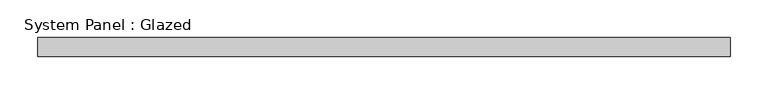
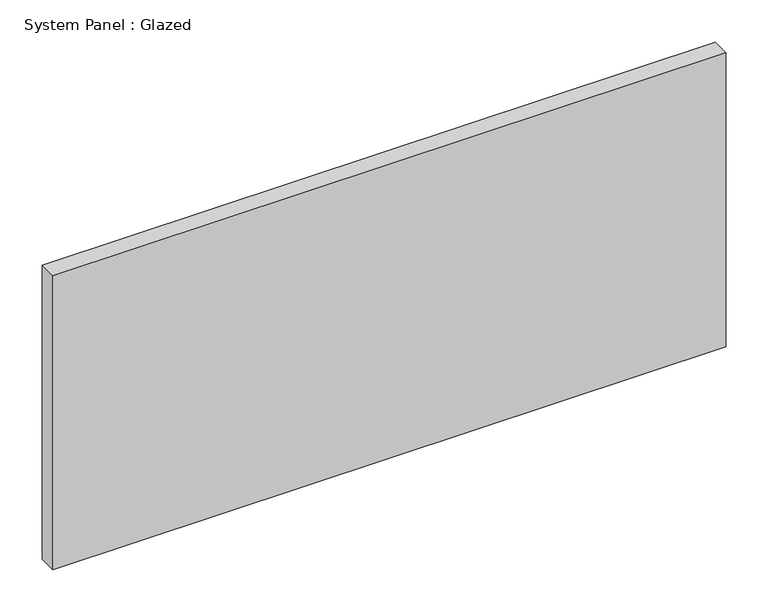
"""IFC4 building model written with IfcOpenShell, lengths in millimetres: plate geometry, System Panel : Glazed."""

from ifc_helpers import new_model, si_unit, origin, origin_with_axes, place, context, project, spatial, polyline, outline, extrude, source, transform, mapped, element, save


def system_panel_glazed_5efa86ec(model_context):
    return source(origin(), model_context, "Body", "SweptSolid", [
        extrude(outline(polyline([(460.375, 19.05), (-460.375, 19.05), (-460.375, 44.45), (460.375, 44.45), (460.375, 19.05)])), origin_with_axes(), (0.0, 0.0, 1.0), 425.45),
    ])


if __name__ == "__main__":
    model = new_model("IFC4")
    model_context = context("Model", 3, world=origin())
    ifc_project = project(units=[si_unit("LENGTHUNIT", "METRE", prefix="MILLI")], contexts=[model_context])
    site = spatial("IfcSite", under=ifc_project)
    building = spatial("IfcBuilding", under=site)
    placement = place(None, origin())
    system_panel_glazed_shape = system_panel_glazed_5efa86ec(model_context)
    element("IfcPlate", 1, ObjectType="System Panel : Glazed", at=placement, inside=building, context=model_context, shape_type="MappedRepresentation", body=[
        mapped(system_panel_glazed_shape, transform((0.0, 0.0, 0.0), x_axis=(1.0, 0.0, 0.0), y_axis=(0.0, 1.0, 0.0), z_axis=(0.0, 0.0, 1.0))),
    ])
    save(model, "model.ifc")

# Revit data of these elements
# Type "System Panel : Glazed"
#   Construction Type Id = "GSP4R"
#   Analytic Construction = "1/8 in Pilkington single glazing"
#   Visual Light Transmittance = 0.9
#   Solar Heat Gain Coefficient = 0.86
#   Heat Transfer Coefficient (U) = 1.18115 BTU/(h·ft²·°F)
#   Define Thermal Properties by = 1
# Element 1 (IfcPlate, "System Panel : Glazed")
#   Materials on its faces: "Glass"
# Materials
#   "Glass": class "Glass", colour RGB 0 128 192, transparency 0.75, Description = "Soda Lime Glass", Cost = 0
